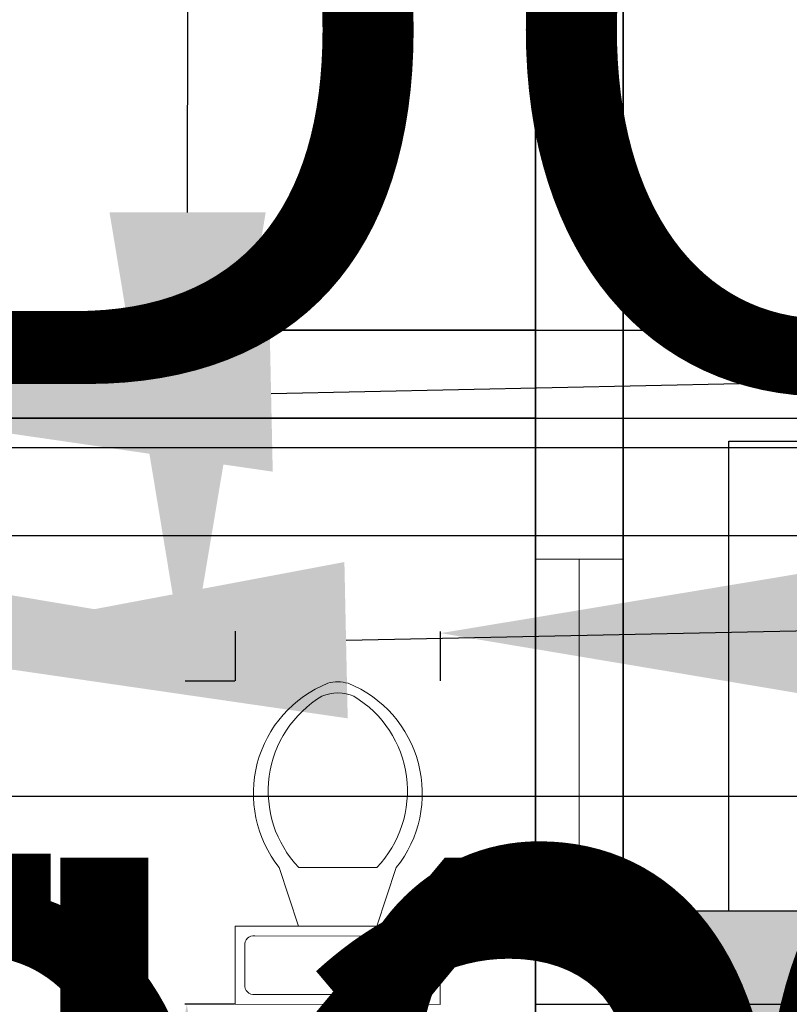
# Model space of a CAD drawing. Units: inches. Extents: x -307 to 2141, y -58 to 895.
# Tile 22 of 28: x 855 to 933, y 481 to 582. Entities that reach past the tile are written whole.
import ezdxf

# ---------------------------------------------------------------- set-up
doc = ezdxf.new("R2010")
doc.units = ezdxf.units.IN
doc.header["$MEASUREMENT"] = 0
for name, color, linetype, lineweight in [('A-ANNO-DIMS', 2, 'Continuous', 18), ('A-FLOR-FIXT', 9, 'Continuous', 18), ('A-GLAZ', 4, 'Continuous', 18), ('A-WALL', 7, 'Continuous', 35)]:
    doc.layers.add(name, color=color, linetype=linetype, lineweight=lineweight)
doc.styles.get("Standard").update_dxf_attribs({"font": 'arial.ttf'})
doc.dimstyles.get("Standard").update_dxf_attribs({"dimtxt": 72, "dimasz": 48, "dimexe": 0.18, "dimexo": 0.0625, "dimgap": 0.09, "dimtad": 0, "dimtih": 1, "dimtoh": 1, "dimdec": 0, "dimrnd": 48, "dimzin": 0, "dimdsep": 46, "dimlunit": 3, "dimtxsty": 'Standard', "dimcen": 0.09, "dimadec": 0, "dimazin": 0, "dimtfac": 1, "dimtdec": 0, "dimtofl": 0, "dimtmove": 0, "dimatfit": 3, "dimfxl": 1, "dimtolj": 1, "dimtzin": 0, "dimarcsym": 0})

# ---------------------------------------------------------------- blocks, each defined once
blk = doc.blocks.new('Toilet - top')
for p, q in [((9.5, -6), (9.5, -2)), ((-8, -8.5), (-8, -8)), ((-7, -8), (-7, -9.5)), ((-4, -8), (-6, -14)), ((4, -8), (6, -14)), ((-10, -8.5), (-8, -8.5)), ((-10, -9.5), (-10, -8.5)), ((-7, -9.5), (-10, -9.5)), ((4, -14), (-4, -14))]:
    blk.add_line(p, q)
blk.add_lwpolyline([(10.5, -8), (10.5, 0), (-10.5, 0), (-10.5, -8)], close=True)
for points in [[(8.5, -1), (-8.5, -1)], [(-9.5, -2), (-9.5, -6)], [(-8.5, -7), (8.5, -7)]]:
    blk.add_lwpolyline(points)
for centre, radius, start, end in [((-8.62, -1.88), 0.884, 81.8699, 188.1301), ((8.62, -1.88), 0.884, 351.8699, 98.1301), ((-8.62, -6.12), 0.884, 171.8699, 278.1301), ((8.62, -6.12), 0.884, 261.8699, 8.1301), ((3.52, -21.58), 12.17, 141.4691, 247.9714), ((4.2, -21.82), 11.33, 136.3677, 238.9468), ((-3.52, -21.58), 12.17, 292.0284, 38.5307), ((-4.2, -21.82), 11.33, 301.053, 43.6321), ((0, -27.88), 4, 245.7318, 294.2682), ((0, -29), 4, 254.8605, 285.1395)]:
    blk.add_arc(centre, radius, start, end)
blk = doc.blocks.new('WIN-36IN')
for p, q in [((0, 36), (9, 36)), ((4.5, 0), (4.5, 36))]:
    blk.add_line(p, q)
blk.add_lwpolyline([(9, 36), (9, 0), (0, 0), (0, 36)])
blk = doc.blocks.new('*D29')
at = {"layer": 'A-ANNO-DIMS', "color": 0, "lineweight": -2, "transparency": 16777216}
for p, q in [((747.42, 450.87), (699.42, 450.87)), ((795.42, 433.61), (795.42, 451.05)), ((882.03, 433.61), (882.03, 451.05)), ((930.03, 450.87), (978.03, 450.87))]:
    blk.add_line(p, q, dxfattribs=at)
at = {"layer": 'A-ANNO-DIMS', "color": 0, "transparency": 16777216}
for points in [[(747.42, 458.87), (747.42, 442.87), (795.42, 450.87)], [(930.03, 458.87), (930.03, 442.87), (882.03, 450.87)]]:
    blk.add_solid(points, dxfattribs=at)
at = {"layer": 'Defpoints', "color": 0, "transparency": 16777216}
for p in [(795.42, 450.87), (795.42, 433.55), (882.03, 433.55)]:
    blk.add_point(p, dxfattribs=at)
at = {"layer": 'A-ANNO-DIMS', "color": 0, "transparency": 16777216, "insert": (647.71, 450.87), "char_height": 72, "attachment_point": 5}
blk.add_mtext('\\A1;87', dxfattribs=at)
blk = doc.blocks.new('*D30')
at = {"layer": 'A-ANNO-DIMS', "color": 0, "lineweight": -2, "transparency": 16777216}
for p, q in [((570.74, 532.83), (570.74, 580.83)), ((570.74, 580.83), (618.74, 580.83)), ((565.4, 484.83), (570.92, 484.83)), ((565.4, 448.83), (570.92, 448.83)), ((570.74, 400.83), (570.74, 352.83))]:
    blk.add_line(p, q, dxfattribs=at)
at = {"layer": 'A-ANNO-DIMS', "color": 0, "transparency": 16777216}
for points in [[(562.74, 532.83), (578.74, 532.83), (570.74, 484.83)], [(562.74, 400.83), (578.74, 400.83), (570.74, 448.83)]]:
    blk.add_solid(points, dxfattribs=at)
at = {"layer": 'Defpoints', "color": 0, "transparency": 16777216}
for p in [(565.34, 484.83), (570.74, 484.83), (565.34, 448.83)]:
    blk.add_point(p, dxfattribs=at)
at = {"layer": 'A-ANNO-DIMS', "color": 0, "transparency": 16777216, "insert": (1030.17, 580.83), "char_height": 72, "attachment_point": 5}
blk.add_mtext('\\A1;WINDOW 36 TYP.', dxfattribs=at)
blk = doc.blocks.new('*D31')
at = {"layer": 'A-ANNO-DIMS', "color": 0, "lineweight": -2, "transparency": 16777216}
for p, q in [((556.34, 448.77), (556.34, 443.25)), ((565.34, 448.77), (565.34, 443.25)), ((508.34, 443.43), (460.34, 443.43)), ((613.34, 443.43), (661.34, 443.43))]:
    blk.add_line(p, q, dxfattribs=at)
at = {"layer": 'A-ANNO-DIMS', "color": 0, "transparency": 16777216}
for points in [[(508.34, 451.43), (508.34, 435.43), (556.34, 443.43)], [(613.34, 451.43), (613.34, 435.43), (565.34, 443.43)]]:
    blk.add_solid(points, dxfattribs=at)
at = {"layer": 'Defpoints', "color": 0, "transparency": 16777216}
for p in [(556.34, 448.83), (565.34, 448.83), (565.34, 443.43)]:
    blk.add_point(p, dxfattribs=at)
at = {"layer": 'A-ANNO-DIMS', "color": 0, "transparency": 16777216, "insert": (808.69, 443.43), "char_height": 72, "attachment_point": 5}
blk.add_mtext('\\A1;9 TYP.', dxfattribs=at)
blk = doc.blocks.new('*D32')
at = {"layer": 'A-ANNO-DIMS', "color": 0, "lineweight": -2, "transparency": 16777216}
for p, q in [((813.29, 682.28), (813.29, 671.36)), ((885.29, 682.28), (885.29, 671.36)), ((765.29, 671.54), (717.29, 671.54)), ((933.29, 671.54), (981.29, 671.54))]:
    blk.add_line(p, q, dxfattribs=at)
at = {"layer": 'A-ANNO-DIMS', "color": 0, "transparency": 16777216}
for points in [[(765.29, 679.54), (765.29, 663.54), (813.29, 671.54)], [(933.29, 679.54), (933.29, 663.54), (885.29, 671.54)]]:
    blk.add_solid(points, dxfattribs=at)
at = {"layer": 'Defpoints', "color": 0, "transparency": 16777216}
for p in [(813.29, 682.34), (885.29, 682.34), (885.29, 671.54)]:
    blk.add_point(p, dxfattribs=at)
at = {"layer": 'A-ANNO-DIMS', "color": 0, "transparency": 16777216, "insert": (1392.73, 671.54), "char_height": 72, "attachment_point": 5}
blk.add_mtext('\\A1;WINDOW 72 TYP.', dxfattribs=at)
blk = doc.blocks.new('*D34')
at = {"layer": 'A-ANNO-DIMS', "color": 0, "lineweight": -2, "transparency": 16777216}
for p, q in [((927.14, 490.97), (927.14, 538.97)), ((927.14, 538.97), (975.14, 538.97)), ((916.4, 442.97), (927.32, 442.97)), ((916.4, 370.95), (927.32, 370.95)), ((927.14, 322.95), (927.14, 274.95))]:
    blk.add_line(p, q, dxfattribs=at)
at = {"layer": 'A-ANNO-DIMS', "color": 0, "transparency": 16777216}
for points in [[(919.14, 490.97), (935.14, 490.97), (927.14, 442.97)], [(919.14, 322.95), (935.14, 322.95), (927.14, 370.95)]]:
    blk.add_solid(points, dxfattribs=at)
at = {"layer": 'Defpoints', "color": 0, "transparency": 16777216}
for p in [(916.34, 442.97), (927.14, 442.97), (916.34, 370.95)]:
    blk.add_point(p, dxfattribs=at)
at = {"layer": 'A-ANNO-DIMS', "color": 0, "transparency": 16777216, "insert": (1584.53, 538.97), "char_height": 72, "attachment_point": 5}
blk.add_mtext('\\A1;PAIRED WINDOW 72 TYP.', dxfattribs=at)
blk = doc.blocks.new('*D35')
at = {"layer": 'A-ANNO-DIMS', "color": 0, "lineweight": -2, "transparency": 16777216}
for p, q in [((859.34, 453.77), (811.34, 453.77)), ((907.34, 443.03), (907.34, 453.95)), ((916.34, 443.03), (916.34, 453.95)), ((964.34, 453.77), (1012.34, 453.77))]:
    blk.add_line(p, q, dxfattribs=at)
at = {"layer": 'A-ANNO-DIMS', "color": 0, "transparency": 16777216}
for points in [[(859.34, 461.77), (859.34, 445.77), (907.34, 453.77)], [(964.34, 461.77), (964.34, 445.77), (916.34, 453.77)]]:
    blk.add_solid(points, dxfattribs=at)
at = {"layer": 'Defpoints', "color": 0, "transparency": 16777216}
for p in [(907.34, 453.77), (907.34, 442.97), (916.34, 442.97)]:
    blk.add_point(p, dxfattribs=at)
at = {"layer": 'A-ANNO-DIMS', "color": 0, "transparency": 16777216, "insert": (663.98, 453.77), "char_height": 72, "attachment_point": 5}
blk.add_mtext('\\A1;9 TYP.', dxfattribs=at)
blk = doc.blocks.new('*D36')
at = {"layer": 'A-ANNO-DIMS', "color": 0, "lineweight": -2, "transparency": 16777216}
for p, q in [((871.71, 562.4), (871.76, 610.4)), ((876.55, 514.4), (871.47, 514.4)), ((876.51, 481.35), (871.44, 481.36)), ((871.56, 433.36), (871.51, 385.36)), ((871.51, 385.36), (823.51, 385.36))]:
    blk.add_line(p, q, dxfattribs=at)
at = {"layer": 'A-ANNO-DIMS', "color": 0, "transparency": 16777216}
for points in [[(863.71, 562.41), (879.71, 562.4), (871.65, 514.4)], [(863.56, 433.37), (879.56, 433.35), (871.62, 481.36)]]:
    blk.add_solid(points, dxfattribs=at)
at = {"layer": 'Defpoints', "color": 0, "transparency": 16777216}
for p in [(876.61, 514.4), (871.62, 481.36), (876.57, 481.35)]:
    blk.add_point(p, dxfattribs=at)
at = {"layer": 'A-ANNO-DIMS', "color": 0, "transparency": 16777216, "insert": (548.95, 385.36), "char_height": 72, "attachment_point": 5}
blk.add_mtext('\\A1;WC 33 TYP.', dxfattribs=at)
blk = doc.blocks.new('*D37')
at = {"layer": 'A-ANNO-DIMS', "color": 0, "lineweight": -2, "transparency": 16777216}
for p, q in [((828.62, 519.41), (780.62, 519.46)), ((876.61, 514.46), (876.62, 519.54)), ((897.61, 514.44), (897.62, 519.51)), ((945.62, 519.28), (993.62, 519.22))]:
    blk.add_line(p, q, dxfattribs=at)
at = {"layer": 'A-ANNO-DIMS', "color": 0, "transparency": 16777216}
for points in [[(828.63, 527.41), (828.61, 511.41), (876.62, 519.36)], [(945.63, 527.28), (945.61, 511.28), (897.62, 519.33)]]:
    blk.add_solid(points, dxfattribs=at)
at = {"layer": 'Defpoints', "color": 0, "transparency": 16777216}
for p in [(876.62, 519.36), (876.61, 514.4), (897.61, 514.38)]:
    blk.add_point(p, dxfattribs=at)
at = {"layer": 'A-ANNO-DIMS', "color": 0, "transparency": 16777216, "insert": (604.68, 519.46), "char_height": 72, "attachment_point": 5}
blk.add_mtext('\\A1;21 TYP.', dxfattribs=at)
blk = doc.blocks.new('*D42')
at = {"layer": 'A-ANNO-DIMS', "color": 0, "lineweight": -2, "transparency": 16777216}
for p, q in [((880.26, 543.86), (928.25, 544.87)), ((822.3, 541.2), (822.27, 542.82)), ((832.3, 541.41), (832.27, 543.03)), ((774.28, 541.63), (726.29, 540.62))]:
    blk.add_line(p, q, dxfattribs=at)
at = {"layer": 'A-ANNO-DIMS', "color": 0, "transparency": 16777216}
for points in [[(880.09, 551.86), (880.43, 535.86), (832.27, 542.85)], [(774.11, 549.63), (774.45, 533.63), (822.27, 542.64)]]:
    blk.add_solid(points, dxfattribs=at)
at = {"layer": 'Defpoints', "color": 0, "transparency": 16777216}
for p in [(832.27, 542.85), (832.3, 541.35), (822.3, 541.14)]:
    blk.add_point(p, dxfattribs=at)
at = {"layer": 'A-ANNO-DIMS', "color": 0, "transparency": 16777216, "insert": (1192.89, 544.87), "char_height": 72, "attachment_point": 5}
blk.add_mtext('\\A1;FAUCET 10', dxfattribs=at)
blk = doc.blocks.new('*D44')
at = {"layer": 'A-ANNO-DIMS', "color": 0, "lineweight": -2, "transparency": 16777216}
for p, q in [((839.87, 521.22), (839.95, 517.42)), ((815.33, 520.71), (815.41, 516.91)), ((887.94, 518.61), (935.93, 519.62)), ((767.41, 516.08), (719.42, 515.07))]:
    blk.add_line(p, q, dxfattribs=at)
at = {"layer": 'A-ANNO-DIMS', "color": 0, "transparency": 16777216}
for points in [[(887.77, 526.61), (888.11, 510.61), (839.95, 517.6)], [(767.25, 524.08), (767.58, 508.08), (815.4, 517.09)]]:
    blk.add_solid(points, dxfattribs=at)
at = {"layer": 'Defpoints', "color": 0, "transparency": 16777216}
for p in [(839.87, 521.29), (815.33, 520.77), (839.95, 517.6)]:
    blk.add_point(p, dxfattribs=at)
at = {"layer": 'A-ANNO-DIMS', "color": 0, "transparency": 16777216, "insert": (1151.16, 519.62), "char_height": 72, "attachment_point": 5}
blk.add_mtext('\\A1;BASIN 25', dxfattribs=at)
blk = doc.blocks.new('*D46')
at = {"layer": 'A-ANNO-DIMS', "color": 0, "lineweight": -2, "transparency": 16777216}
for p, q in [((801.41, 645.78), (801.41, 642.52)), ((822.41, 645.78), (822.41, 642.52)), ((753.41, 642.7), (705.41, 642.7)), ((870.41, 642.7), (918.41, 642.7))]:
    blk.add_line(p, q, dxfattribs=at)
at = {"layer": 'A-ANNO-DIMS', "color": 0, "transparency": 16777216}
for points in [[(753.41, 650.7), (753.41, 634.7), (801.41, 642.7)], [(870.41, 650.7), (870.41, 634.7), (822.41, 642.7)]]:
    blk.add_solid(points, dxfattribs=at)
at = {"layer": 'Defpoints', "color": 0, "transparency": 16777216}
for p in [(801.41, 645.85), (822.41, 645.85), (822.41, 642.7)]:
    blk.add_point(p, dxfattribs=at)
at = {"layer": 'A-ANNO-DIMS', "color": 0, "transparency": 16777216, "insert": (1282.7, 642.7), "char_height": 72, "attachment_point": 5}
blk.add_mtext('\\A1;DESK CHAIR 21', dxfattribs=at)
blk = doc.blocks.new('*D47')
at = {"layer": 'A-ANNO-DIMS', "color": 0, "lineweight": -2, "transparency": 16777216}
for p, q in [((825.56, 711.18), (825.56, 759.18)), ((825.56, 759.18), (873.56, 759.18)), ((822.48, 663.18), (825.74, 663.18)), ((822.48, 645.85), (825.74, 645.85)), ((825.56, 597.85), (825.56, 549.85))]:
    blk.add_line(p, q, dxfattribs=at)
at = {"layer": 'A-ANNO-DIMS', "color": 0, "transparency": 16777216}
for points in [[(817.56, 711.18), (833.56, 711.18), (825.56, 663.18)], [(817.56, 597.85), (833.56, 597.85), (825.56, 645.85)]]:
    blk.add_solid(points, dxfattribs=at)
at = {"layer": 'Defpoints', "color": 0, "transparency": 16777216}
for p in [(822.41, 663.18), (825.56, 663.18), (822.41, 645.85)]:
    blk.add_point(p, dxfattribs=at)
at = {"layer": 'A-ANNO-DIMS', "color": 0, "transparency": 16777216, "insert": (921.83, 759.18), "char_height": 72, "attachment_point": 5}
blk.add_mtext('\\A1;17', dxfattribs=at)
blk = doc.blocks.new('*D52')
at = {"layer": 'A-ANNO-DIMS', "color": 0, "lineweight": -2, "transparency": 16777216}
for p, q in [((660.21, 554.25), (660.21, 602.25)), ((673.8, 506.25), (660.03, 506.25)), ((673.8, 415.25), (660.03, 415.25)), ((660.21, 367.25), (660.21, 319.25))]:
    blk.add_line(p, q, dxfattribs=at)
at = {"layer": 'A-ANNO-DIMS', "color": 0, "transparency": 16777216}
for points in [[(652.21, 554.25), (668.21, 554.25), (660.21, 506.25)], [(652.21, 367.25), (668.21, 367.25), (660.21, 415.25)]]:
    blk.add_solid(points, dxfattribs=at)
at = {"layer": 'Defpoints', "color": 0, "transparency": 16777216}
for p in [(673.86, 506.25), (660.21, 415.25), (673.86, 415.25)]:
    blk.add_point(p, dxfattribs=at)
at = {"layer": 'A-ANNO-DIMS', "color": 0, "transparency": 16777216, "insert": (660.21, 460.75), "char_height": 72, "attachment_point": 5}
blk.add_mtext('\\A1;DINING SET 91', dxfattribs=at)
blk = doc.blocks.new('*D54')
at = {"layer": 'A-ANNO-DIMS', "color": 0, "lineweight": -2, "transparency": 16777216}
for p, q in [((605.34, 412.35), (605.34, 460.35)), ((605.34, 460.35), (653.34, 460.35)), ((596.4, 364.35), (605.52, 364.35)), ((596.4, 304.35), (605.52, 304.35)), ((605.34, 256.35), (605.34, 208.35))]:
    blk.add_line(p, q, dxfattribs=at)
at = {"layer": 'A-ANNO-DIMS', "color": 0, "transparency": 16777216}
for points in [[(597.34, 412.35), (613.34, 412.35), (605.34, 364.35)], [(597.34, 256.35), (613.34, 256.35), (605.34, 304.35)]]:
    blk.add_solid(points, dxfattribs=at)
at = {"layer": 'Defpoints', "color": 0, "transparency": 16777216}
for p in [(596.34, 364.35), (605.34, 364.35), (596.34, 304.35)]:
    blk.add_point(p, dxfattribs=at)
at = {"layer": 'A-ANNO-DIMS', "color": 0, "transparency": 16777216, "insert": (854, 460.35), "char_height": 72, "attachment_point": 5}
blk.add_mtext('\\A1;DESK 60', dxfattribs=at)
blk = doc.blocks.new('*D56')
at = {"layer": 'A-ANNO-DIMS', "color": 0, "lineweight": -2, "transparency": 16777216}
for p, q in [((679.73, 723.21), (679.73, 771.21)), ((679.73, 771.21), (727.73, 771.21)), ((675.74, 675.21), (679.91, 675.21)), ((675.74, 648.21), (679.91, 648.21)), ((679.73, 600.21), (679.73, 552.21))]:
    blk.add_line(p, q, dxfattribs=at)
at = {"layer": 'A-ANNO-DIMS', "color": 0, "transparency": 16777216}
for points in [[(671.73, 723.21), (687.73, 723.21), (679.73, 675.21)], [(671.73, 600.21), (687.73, 600.21), (679.73, 648.21)]]:
    blk.add_solid(points, dxfattribs=at)
at = {"layer": 'Defpoints', "color": 0, "transparency": 16777216}
for p in [(675.68, 675.21), (679.73, 675.21), (675.68, 648.21)]:
    blk.add_point(p, dxfattribs=at)
at = {"layer": 'A-ANNO-DIMS', "color": 0, "transparency": 16777216, "insert": (1006.66, 771.21), "char_height": 72, "attachment_point": 5}
blk.add_mtext('\\A1;ROCKER 27', dxfattribs=at)
blk = doc.blocks.new('*D62')
at = {"layer": 'A-ANNO-DIMS', "color": 0, "lineweight": -2, "transparency": 16777216}
for p, q in [((556.34, 691.4), (556.34, 722.72)), ((916.34, 490.97), (916.34, 722.72)), ((604.34, 722.54), (656.85, 722.54)), ((868.34, 722.54), (815.82, 722.54))]:
    blk.add_line(p, q, dxfattribs=at)
at = {"layer": 'A-ANNO-DIMS', "color": 0, "transparency": 16777216}
for points in [[(604.34, 730.54), (604.34, 714.54), (556.34, 722.54)], [(868.34, 730.54), (868.34, 714.54), (916.34, 722.54)]]:
    blk.add_solid(points, dxfattribs=at)
at = {"layer": 'Defpoints', "color": 0, "transparency": 16777216}
for p in [(916.34, 722.54), (556.34, 691.34), (916.34, 490.9)]:
    blk.add_point(p, dxfattribs=at)
at = {"layer": 'A-ANNO-DIMS', "color": 0, "transparency": 16777216, "insert": (736.34, 722.54), "char_height": 72, "attachment_point": 5}
blk.add_mtext('\\A1;360', dxfattribs=at)
blk = doc.blocks.new('*D63')
at = {"layer": 'A-ANNO-DIMS', "color": 0, "lineweight": -2, "transparency": 16777216}
for p, q in [((916.4, 691.34), (947.72, 691.34)), ((947.54, 643.34), (947.54, 416.19)), ((947.54, 115.34), (947.54, 342.49)), ((704.68, 67.34), (947.72, 67.34))]:
    blk.add_line(p, q, dxfattribs=at)
at = {"layer": 'A-ANNO-DIMS', "color": 0, "transparency": 16777216}
for points in [[(939.54, 643.34), (955.54, 643.34), (947.54, 691.34)], [(939.54, 115.34), (955.54, 115.34), (947.54, 67.34)]]:
    blk.add_solid(points, dxfattribs=at)
at = {"layer": 'Defpoints', "color": 0, "transparency": 16777216}
for p in [(916.34, 691.34), (704.62, 67.34), (947.54, 67.34)]:
    blk.add_point(p, dxfattribs=at)
at = {"layer": 'A-ANNO-DIMS', "color": 0, "transparency": 16777216, "insert": (947.54, 379.34), "char_height": 72, "attachment_point": 5}
blk.add_mtext('\\A1;624', dxfattribs=at)
blk = doc.blocks.new('*D78')
at = {"layer": 'A-ANNO-DIMS', "color": 0, "lineweight": -2, "transparency": 16777216}
for p, q in [((947.53984, 730.340828), (947.53984, 778.340828)), ((778.39834, 682.340828), (947.71984, 682.340828)), ((730.39834, 598.340828), (947.71984, 598.340828)), ((947.53984, 550.340828), (947.53984, 502.340828))]:
    blk.add_line(p, q, dxfattribs=at)
at = {"layer": 'A-ANNO-DIMS', "color": 0, "transparency": 16777216}
for points in [[(939.53984, 730.340828), (955.53984, 730.340828), (947.53984, 682.340828)], [(939.53984, 550.340828), (955.53984, 550.340828), (947.53984, 598.340828)]]:
    blk.add_solid(points, dxfattribs=at)
at = {"layer": 'Defpoints', "color": 0, "transparency": 16777216}
for p in [(778.33584, 682.340828), (947.53984, 682.340828), (730.33584, 598.340828)]:
    blk.add_point(p, dxfattribs=at)
at = {"layer": 'A-ANNO-DIMS', "color": 0, "transparency": 16777216, "insert": (947.53984, 640.340828), "char_height": 72, "attachment_point": 5}
blk.add_mtext('\\A1;84', dxfattribs=at)
blk = doc.blocks.new('*D79')
at = {"layer": 'A-ANNO-DIMS', "color": 0, "lineweight": -2, "transparency": 16777216}
for p, q in [((947.54, 682.34), (947.54, 730.34)), ((947.54, 730.34), (995.54, 730.34)), ((907.4, 682.34), (947.72, 682.34)), ((947.54, 598.34), (947.54, 634.34)), ((907.4, 550.34), (947.72, 550.34))]:
    blk.add_line(p, q, dxfattribs=at)
at = {"layer": 'A-ANNO-DIMS', "color": 0, "transparency": 16777216}
for points in [[(939.54, 634.34), (955.54, 634.34), (947.54, 682.34)], [(939.54, 598.34), (955.54, 598.34), (947.54, 550.34)]]:
    blk.add_solid(points, dxfattribs=at)
at = {"layer": 'Defpoints', "color": 0, "transparency": 16777216}
for p in [(907.34, 682.34), (947.54, 682.34), (907.34, 550.34)]:
    blk.add_point(p, dxfattribs=at)
at = {"layer": 'A-ANNO-DIMS', "color": 0, "transparency": 16777216, "insert": (1071.41, 730.34), "char_height": 72, "attachment_point": 5}
blk.add_mtext('\\A1;132', dxfattribs=at)
blk = doc.blocks.new('*D80')
at = {"layer": 'A-ANNO-DIMS', "color": 0, "lineweight": -2, "transparency": 16777216}
for p, q in [((811.34, 517.4), (811.34, 722.72)), ((907.34, 541.4), (907.34, 722.72)), ((763.34, 722.54), (715.34, 722.54)), ((955.34, 722.54), (1003.34, 722.54))]:
    blk.add_line(p, q, dxfattribs=at)
at = {"layer": 'A-ANNO-DIMS', "color": 0, "transparency": 16777216}
for points in [[(763.34, 730.54), (763.34, 714.54), (811.34, 722.54)], [(955.34, 730.54), (955.34, 714.54), (907.34, 722.54)]]:
    blk.add_solid(points, dxfattribs=at)
at = {"layer": 'Defpoints', "color": 0, "transparency": 16777216}
for p in [(907.34, 722.54), (907.34, 541.34), (811.34, 517.34)]:
    blk.add_point(p, dxfattribs=at)
at = {"layer": 'A-ANNO-DIMS', "color": 0, "transparency": 16777216, "insert": (1054.97, 722.54), "char_height": 72, "attachment_point": 5}
blk.add_mtext('\\A1;96', dxfattribs=at)
blk = doc.blocks.new('*D81')
at = {"layer": 'A-ANNO-DIMS', "color": 0, "lineweight": -2, "transparency": 16777216}
for p, q in [((947.54, 589.34), (947.54, 637.34)), ((947.54, 637.34), (995.54, 637.34)), ((907.4, 541.34), (947.72, 541.34)), ((907.4, 481.34), (947.72, 481.34)), ((947.54, 433.34), (947.54, 385.34))]:
    blk.add_line(p, q, dxfattribs=at)
at = {"layer": 'A-ANNO-DIMS', "color": 0, "transparency": 16777216}
for points in [[(939.54, 589.34), (955.54, 589.34), (947.54, 541.34)], [(939.54, 433.34), (955.54, 433.34), (947.54, 481.34)]]:
    blk.add_solid(points, dxfattribs=at)
at = {"layer": 'Defpoints', "color": 0, "transparency": 16777216}
for p in [(907.34, 541.34), (947.54, 541.34), (907.34, 481.34)]:
    blk.add_point(p, dxfattribs=at)
at = {"layer": 'A-ANNO-DIMS', "color": 0, "transparency": 16777216, "insert": (1047.27, 637.34), "char_height": 72, "attachment_point": 5}
blk.add_mtext('\\A1;60', dxfattribs=at)
blk = doc.blocks.new('*D83')
at = {"layer": 'A-ANNO-DIMS', "color": 0, "lineweight": -2, "transparency": 16777216}
for p, q in [((947.54, 538.9), (947.54, 586.9)), ((916.4, 490.9), (947.72, 490.9)), ((907.4, 481.34), (947.72, 481.34)), ((947.54, 433.34), (947.54, 385.34)), ((947.54, 385.34), (899.54, 385.34))]:
    blk.add_line(p, q, dxfattribs=at)
at = {"layer": 'A-ANNO-DIMS', "color": 0, "transparency": 16777216}
for points in [[(939.54, 538.9), (955.54, 538.9), (947.54, 490.9)], [(939.54, 433.34), (955.54, 433.34), (947.54, 481.34)]]:
    blk.add_solid(points, dxfattribs=at)
at = {"layer": 'Defpoints', "color": 0, "transparency": 16777216}
for p in [(916.34, 490.9), (907.34, 481.34), (947.54, 481.34)]:
    blk.add_point(p, dxfattribs=at)
at = {"layer": 'A-ANNO-DIMS', "color": 0, "transparency": 16777216, "insert": (777.97, 385.34), "char_height": 72, "attachment_point": 5}
blk.add_mtext('\\A1;9.563', dxfattribs=at)
blk = doc.blocks.new('*D85')
at = {"layer": 'A-ANNO-DIMS', "color": 0, "lineweight": -2, "transparency": 16777216}
for p, q in [((947.54, 472.34), (947.54, 520.34)), ((947.54, 520.34), (995.54, 520.34)), ((907.4, 472.34), (947.72, 472.34)), ((947.54, 364.34), (947.54, 424.34)), ((916.4, 316.34), (947.72, 316.34))]:
    blk.add_line(p, q, dxfattribs=at)
at = {"layer": 'A-ANNO-DIMS', "color": 0, "transparency": 16777216}
for points in [[(939.54, 424.34), (955.54, 424.34), (947.54, 472.34)], [(939.54, 364.34), (955.54, 364.34), (947.54, 316.34)]]:
    blk.add_solid(points, dxfattribs=at)
at = {"layer": 'Defpoints', "color": 0, "transparency": 16777216}
for p in [(907.34, 472.34), (947.54, 472.34), (916.34, 316.34)]:
    blk.add_point(p, dxfattribs=at)
at = {"layer": 'A-ANNO-DIMS', "color": 0, "transparency": 16777216, "insert": (1071.76, 520.34), "char_height": 72, "attachment_point": 5}
blk.add_mtext('\\A1;156', dxfattribs=at)
blk = doc.blocks.new('*D94')
at = {"layer": 'A-ANNO-DIMS', "color": 0, "lineweight": -2, "transparency": 16777216}
for p, q in [((565.34, 529.4), (565.34, 722.72)), ((629.84, 529.4), (629.84, 722.72)), ((517.34, 722.54), (469.34, 722.54)), ((677.84, 722.54), (725.84, 722.54))]:
    blk.add_line(p, q, dxfattribs=at)
at = {"layer": 'A-ANNO-DIMS', "color": 0, "transparency": 16777216}
for points in [[(517.34, 730.54), (517.34, 714.54), (565.34, 722.54)], [(677.84, 730.54), (677.84, 714.54), (629.84, 722.54)]]:
    blk.add_solid(points, dxfattribs=at)
at = {"layer": 'Defpoints', "color": 0, "transparency": 16777216}
for p in [(629.84, 722.54), (565.34, 529.34), (629.84, 529.34)]:
    blk.add_point(p, dxfattribs=at)
at = {"layer": 'A-ANNO-DIMS', "color": 0, "transparency": 16777216, "insert": (819.9, 722.54), "char_height": 72, "attachment_point": 5}
blk.add_mtext('\\A1;64.5', dxfattribs=at)
blk = doc.blocks.new('*D95')
at = {"layer": 'A-ANNO-DIMS', "color": 0, "lineweight": -2, "transparency": 16777216}
for p, q in [((947.54, 577.34), (947.54, 625.34)), ((947.54, 625.34), (995.54, 625.34)), ((629.9, 529.34), (947.72, 529.34)), ((629.9, 502.66), (947.72, 502.66)), ((947.54, 454.66), (947.54, 406.66))]:
    blk.add_line(p, q, dxfattribs=at)
at = {"layer": 'A-ANNO-DIMS', "color": 0, "transparency": 16777216}
for points in [[(939.54, 577.34), (955.54, 577.34), (947.54, 529.34)], [(939.54, 454.66), (955.54, 454.66), (947.54, 502.66)]]:
    blk.add_solid(points, dxfattribs=at)
at = {"layer": 'Defpoints', "color": 0, "transparency": 16777216}
for p in [(629.84, 529.34), (947.54, 529.34), (629.84, 502.66)]:
    blk.add_point(p, dxfattribs=at)
at = {"layer": 'A-ANNO-DIMS', "color": 0, "transparency": 16777216, "insert": (1117.8, 625.34), "char_height": 72, "attachment_point": 5}
blk.add_mtext('\\A1;26.68', dxfattribs=at)
blk = doc.blocks.new('*D97')
at = {"layer": 'A-ANNO-DIMS', "color": 0, "lineweight": -2, "transparency": 16777216}
for p, q in [((947.54, 637.34), (947.54, 685.34)), ((947.54, 685.34), (995.54, 685.34)), ((685.4, 589.34), (947.72, 589.34)), ((685.4, 538.34), (947.72, 538.34)), ((947.54, 490.34), (947.54, 442.34))]:
    blk.add_line(p, q, dxfattribs=at)
at = {"layer": 'A-ANNO-DIMS', "color": 0, "transparency": 16777216}
for points in [[(939.54, 637.34), (955.54, 637.34), (947.54, 589.34)], [(939.54, 490.34), (955.54, 490.34), (947.54, 538.34)]]:
    blk.add_solid(points, dxfattribs=at)
at = {"layer": 'Defpoints', "color": 0, "transparency": 16777216}
for p in [(685.34, 589.34), (947.54, 589.34), (685.34, 538.34)]:
    blk.add_point(p, dxfattribs=at)
at = {"layer": 'A-ANNO-DIMS', "color": 0, "transparency": 16777216, "insert": (1040.25, 685.34), "char_height": 72, "attachment_point": 5}
blk.add_mtext('\\A1;51', dxfattribs=at)
blk = doc.blocks.new('*D104')
at = {"layer": 'A-ANNO-DIMS', "color": 0, "lineweight": -2, "transparency": 16777216}
for p, q in [((885.13, 418.95), (885.13, 466.95)), ((885.13, 466.95), (933.13, 466.95)), ((916.27, 370.95), (884.95, 370.95)), ((916.27, 307.34), (884.95, 307.34)), ((885.13, 259.34), (885.13, 211.34))]:
    blk.add_line(p, q, dxfattribs=at)
at = {"layer": 'A-ANNO-DIMS', "color": 0, "transparency": 16777216}
for points in [[(877.13, 418.95), (893.13, 418.95), (885.13, 370.95)], [(877.13, 259.34), (893.13, 259.34), (885.13, 307.34)]]:
    blk.add_solid(points, dxfattribs=at)
at = {"layer": 'Defpoints', "color": 0, "transparency": 16777216}
for p in [(885.13, 370.95), (916.34, 370.95), (916.34, 307.34)]:
    blk.add_point(p, dxfattribs=at)
at = {"layer": 'A-ANNO-DIMS', "color": 0, "transparency": 16777216, "insert": (1047.95, 466.95), "char_height": 72, "attachment_point": 5}
blk.add_mtext('\\A1;63.61', dxfattribs=at)
blk = doc.blocks.new('*D107')
at = {"layer": 'A-ANNO-DIMS', "color": 0, "lineweight": -2, "transparency": 16777216}
for p, q in [((565.34, 409.4), (565.34, 722.72)), ((589.34, 409.4), (589.34, 722.72)), ((517.34, 722.54), (469.34, 722.54)), ((637.34, 722.54), (685.34, 722.54))]:
    blk.add_line(p, q, dxfattribs=at)
at = {"layer": 'A-ANNO-DIMS', "color": 0, "transparency": 16777216}
for points in [[(517.34, 730.54), (517.34, 714.54), (565.34, 722.54)], [(637.34, 730.54), (637.34, 714.54), (589.34, 722.54)]]:
    blk.add_solid(points, dxfattribs=at)
at = {"layer": 'Defpoints', "color": 0, "transparency": 16777216}
for p in [(589.34, 722.54), (565.34, 409.34), (589.34, 409.34)]:
    blk.add_point(p, dxfattribs=at)
at = {"layer": 'A-ANNO-DIMS', "color": 0, "transparency": 16777216, "insert": (835.49, 722.54), "char_height": 72, "attachment_point": 5}
blk.add_mtext('\\A1;24.003', dxfattribs=at)
blk = doc.blocks.new('*D108')
at = {"layer": 'A-ANNO-DIMS', "color": 0, "lineweight": -2, "transparency": 16777216}
for p, q in [((947.54, 550.66), (947.54, 598.66)), ((589.4, 502.66), (947.72, 502.66)), ((589.4, 409.34), (947.72, 409.34)), ((947.54, 361.34), (947.54, 313.34))]:
    blk.add_line(p, q, dxfattribs=at)
at = {"layer": 'A-ANNO-DIMS', "color": 0, "transparency": 16777216}
for points in [[(939.54, 550.66), (955.54, 550.66), (947.54, 502.66)], [(939.54, 361.34), (955.54, 361.34), (947.54, 409.34)]]:
    blk.add_solid(points, dxfattribs=at)
at = {"layer": 'Defpoints', "color": 0, "transparency": 16777216}
for p in [(589.34, 502.66), (947.54, 502.66), (589.34, 409.34)]:
    blk.add_point(p, dxfattribs=at)
at = {"layer": 'A-ANNO-DIMS', "color": 0, "transparency": 16777216, "insert": (947.54, 456), "char_height": 72, "attachment_point": 5}
blk.add_mtext('\\A1;93.32', dxfattribs=at)

msp = doc.modelspace()

# ---------------------------------------------------------------- linework, layer by layer
at = {"layer": 'A-WALL'}
for p, q in [((916.3358, 166.3408), (916.3358, 691.3408)), ((907.3358, 166.3408), (907.3358, 682.3408)), ((907.3358, 550.3408), (778.3358, 550.3408)), ((907.3358, 541.3408), (778.3358, 541.3408))]:
    msp.add_line(p, q, dxfattribs=at)

# ---------------------------------------------------------------- block references
at = {"layer": 'A-FLOR-FIXT', "rotation": 179.9358923931402}
msp.add_blockref('Toilet - top', (887.0736, 481.3408), dxfattribs=at)
at = {"layer": 'A-GLAZ'}
msp.add_blockref('WIN-36IN', (907.336, 490.9038), dxfattribs=at)

# ---------------------------------------------------------------- dimensions: what is measured, and where the dimension line sits
at = {"layer": 'A-ANNO-DIMS'}
for base, p1, p2, angle, text, picture, middle in [((679.7317, 675.211), (675.6817, 648.211), (675.6817, 675.211), 90, 'ROCKER <>', '*D56', (1006.6621, 771.211)), ((927.1381, 442.9669), (916.3358, 370.9517), (916.3358, 442.9669), 90, 'PAIRED WINDOW <> TYP.', '*D34', (1584.5269, 538.9669)), ((570.7358, 484.8333), (565.3358, 448.8333), (565.3358, 484.8333), 90, 'WINDOW <> TYP.', '*D30', (1030.1737, 580.8333)), ((832.2692, 542.8502), (822.3029, 541.1403), (832.3007, 541.3505), 1.204628, 'FAUCET <>', '*D42', (1192.8864, 544.8684)), ((660.2083, 415.2485), (673.8583, 506.2485), (673.8583, 415.2485), 270, 'DINING SET <>', '*D52', (660.2083, 460.7485)), ((839.9481, 517.6035), (815.3253, 520.7692), (839.8707, 521.2853), 1.204628, 'BASIN <>', '*D44', (1151.1574, 519.6217)), ((876.6162, 519.3557), (897.6106, 514.3753), (876.6106, 514.3988), 179.935892, '<> TYP.', '*D37', (604.6763, 519.4631)), ((871.6167, 481.3581), (876.6106, 514.3988), (876.5736, 481.3526), 269.935892, 'WC <> TYP.', '*D36', (548.95, 385.3582)), ((605.3358, 364.3488), (596.3358, 304.3488), (596.3358, 364.3488), 90, 'DESK <>', '*D54', (854.0043, 460.3488)), ((907.3358, 453.7692), (916.3358, 442.9669), (907.3358, 442.9669), 180, '<> TYP.', '*D35', (663.9798, 453.7692))]:
    dim = msp.add_linear_dim(base=base, p1=p1, p2=p2, angle=angle, text=text, dimstyle='Standard', override={"dimdec": 0, "dimlfac": 1, "dimrnd": 0, "dimzin": 0, "dimdsep": 46, "dimlunit": 2}, dxfattribs=at)
    dim.commit()
    dim.dimension.update_dxf_attribs({"geometry": picture, "text_midpoint": middle})
for base, p1, p2, text, picture, middle in [((885.2934, 671.5408), (813.2934, 682.3408), (885.2934, 682.3408), 'WINDOW <> TYP.', '*D32', (1392.7312, 671.5408)), ((822.4132, 642.696), (801.4132, 645.846), (822.4132, 645.846), 'DESK CHAIR <>', '*D46', (1282.7024, 642.696)), ((565.3358, 443.4333), (556.3358, 448.8333), (565.3358, 448.8333), '<> TYP.', '*D31', (808.6919, 443.4333))]:
    dim = msp.add_linear_dim(base=base, p1=p1, p2=p2, text=text, dimstyle='Standard', override={"dimdec": 0, "dimlfac": 1, "dimrnd": 0, "dimzin": 0, "dimdsep": 46, "dimlunit": 2}, dxfattribs=at)
    dim.commit()
    dim.dimension.update_dxf_attribs({"geometry": picture, "text_midpoint": middle})
for base, p1, p2, angle, override, picture, middle in [((825.5632, 663.1793), (822.4132, 645.846), (822.4132, 663.1793), 90, {"dimdec": 0, "dimlfac": 1, "dimrnd": 0, "dimzin": 0, "dimdsep": 46, "dimlunit": 2}, '*D47', (921.8333, 759.1793)), ((947.5398, 682.3408), (730.3358, 598.3408), (778.3358, 682.3408), 90, {"dimdec": 0, "dimlfac": 1, "dimrnd": 0, "dimzin": 0, "dimdsep": 46, "dimlunit": 2}, '*D78', (947.5398, 640.3408)), ((947.5398, 682.3408), (907.3358, 550.3408), (907.3358, 682.3408), 90, {"dimdec": 0, "dimlfac": 1, "dimrnd": 0, "dimzin": 0, "dimdsep": 46, "dimlunit": 2}, '*D79', (1071.4116, 730.3408)), ((947.5398, 589.3408), (685.3358, 538.3408), (685.3358, 589.3408), 90, {"dimdec": 0, "dimlfac": 1, "dimrnd": 0, "dimzin": 0, "dimdsep": 46, "dimlunit": 2}, '*D97', (1040.2492, 685.3408)), ((947.5398, 67.3408), (916.3358, 691.3408), (704.6211, 67.3408), 90, {"dimdec": 0, "dimlfac": 1, "dimrnd": 0, "dimzin": 0, "dimdsep": 46, "dimlunit": 2}, '*D63', (947.5398, 379.3408)), ((947.5398, 541.3408), (907.3358, 481.3408), (907.3358, 541.3408), 90, {"dimdec": 0, "dimlfac": 1, "dimrnd": 0, "dimzin": 0, "dimdsep": 46, "dimlunit": 2}, '*D81', (1047.2724, 637.3408)), ((947.5398, 529.3408), (629.8358, 502.6632), (629.8358, 529.3408), 90, {"dimdec": 2, "dimlfac": 1, "dimrnd": 0, "dimzin": 0, "dimdsep": 46, "dimlunit": 2}, '*D95', (1117.799, 625.3408)), ((947.5398, 502.6632), (589.339, 409.3408), (589.339, 502.6632), 90, {"dimdec": 2, "dimlfac": 1, "dimrnd": 0, "dimzin": 0, "dimdsep": 46, "dimlunit": 2}, '*D108', (947.5398, 456.002)), ((947.5398, 481.3408), (916.3358, 490.9034), (907.3358, 481.3408), 90, {"dimdec": 3, "dimlfac": 1, "dimrnd": 0, "dimzin": 0, "dimdsep": 46, "dimlunit": 2}, '*D83', (777.9683, 385.3408)), ((947.5398, 472.3408), (916.3358, 316.3408), (907.3358, 472.3408), 90, {"dimdec": 0, "dimlfac": 1, "dimrnd": 0, "dimzin": 0, "dimdsep": 46, "dimlunit": 2}, '*D85', (1071.7554, 520.3408)), ((885.1318, 370.9517), (916.3358, 307.3408), (916.3358, 370.9517), 90, {"dimdec": 2, "dimlfac": 1, "dimrnd": 0, "dimzin": 0, "dimdsep": 46, "dimlunit": 2}, '*D104', (1047.9504, 466.9517)), ((795.4208, 450.8711), (882.0282, 433.5496), (795.4208, 433.5496), 180, {"dimdec": 0, "dimlfac": 1, "dimrnd": 0, "dimzin": 0, "dimdsep": 46, "dimlunit": 2}, '*D29', (647.7128, 450.8711))]:
    dim = msp.add_linear_dim(base=base, p1=p1, p2=p2, angle=angle, dimstyle='Standard', override=override, dxfattribs=at)
    dim.commit()
    dim.dimension.update_dxf_attribs({"geometry": picture, "text_midpoint": middle})
for base, p1, p2, override, picture, middle in [((629.8358, 722.5448), (565.3358, 529.3408), (629.8358, 529.3408), {"dimdec": 1, "dimlfac": 1, "dimrnd": 0, "dimzin": 0, "dimdsep": 46, "dimlunit": 2}, '*D94', (819.904, 722.5448)), ((589.339, 722.5448), (565.3358, 409.3408), (589.339, 409.3408), {"dimdec": 3, "dimlfac": 1, "dimrnd": 0, "dimzin": 0, "dimdsep": 46, "dimlunit": 2}, '*D107', (835.4945, 722.5448)), ((916.3358, 722.5448), (556.3358, 691.3408), (916.3358, 490.9034), {"dimdec": 0, "dimlfac": 1, "dimrnd": 0, "dimzin": 0, "dimdsep": 46, "dimlunit": 2}, '*D62', (736.3358, 722.5448)), ((907.3358, 722.5448), (811.3358, 517.3408), (907.3358, 541.3408), {"dimdec": 0, "dimlfac": 1, "dimrnd": 0, "dimzin": 0, "dimdsep": 46, "dimlunit": 2}, '*D80', (1054.9702, 722.5448))]:
    dim = msp.add_linear_dim(base=base, p1=p1, p2=p2, dimstyle='Standard', override=override, dxfattribs=at)
    dim.commit()
    dim.dimension.update_dxf_attribs({"geometry": picture, "text_midpoint": middle})

doc.saveas('drawing.dxf')
